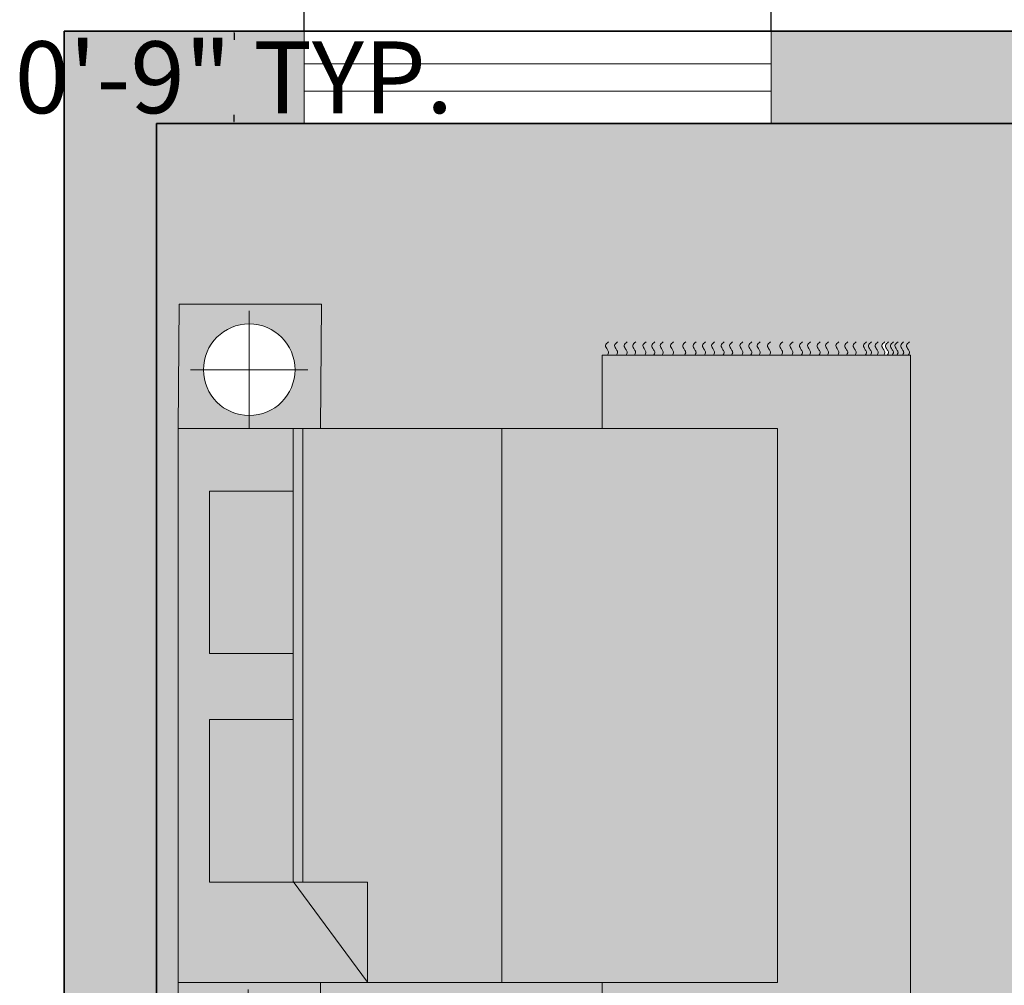
# Model space of a CAD drawing. Units: inches. Extents: x 1316 to 1777, y 813 to 1650.
# Tile 12 of 22: x 1373 to 1469, y 1482 to 1576. Entities that reach past the tile are written whole.
import ezdxf

# ---------------------------------------------------------------- set-up
doc = ezdxf.new("R2010")
doc.units = ezdxf.units.IN
doc.header["$MEASUREMENT"] = 0
for name, color, linetype, lineweight in [('A-ANNO-DIMS', 2, 'Continuous', 18), ('A-FURN-PATT', 23, 'Continuous', 13), ('A-WALL-PATT', 250, 'Continuous', 13), ('furniture', 23, 'Continuous', 18), ('walls', 250, 'Continuous', 35), ('windows', 141, 'Continuous', 18)]:
    doc.layers.add(name, color=color, linetype=linetype, lineweight=lineweight)
doc.layers.add('A-FLOR-PATT', color=254, linetype='Continuous', lineweight=13, true_color=0xfeeab9)
doc.styles.get("Standard").update_dxf_attribs({"font": 'arial.ttf'})
doc.dimstyles.get("Standard").update_dxf_attribs({"dimtxt": 7, "dimasz": 0.18, "dimexe": 0.18, "dimexo": 0.0625, "dimgap": 0.09, "dimtad": 0, "dimtih": 1, "dimtoh": 1, "dimzin": 0, "dimdsep": 46, "dimlunit": 3, "dimtxsty": 'Standard', "dimcen": 0.09, "dimadec": 0, "dimazin": 0, "dimtfac": 1, "dimtofl": 0, "dimtmove": 0, "dimatfit": 3, "dimfxl": 1, "dimtolj": 1, "dimtzin": 0, "dimarcsym": 0})

# ---------------------------------------------------------------- blocks, each defined once
blk = doc.blocks.new('CARPET')
at = {"layer": 'furniture'}
for p, q in [((-51.53, -98.11), (-51.53, -55.12)), ((-51.53, -55.12), (-41.27, -55.12)), ((36, -55.12), (51.55, -55.12)), ((51.55, -55.12), (51.55, -98.11)), ((51.55, -98.11), (-51.53, -98.11))]:
    blk.add_line(p, q, dxfattribs=at)
for points, knots in [([(-53.37, -55.99), (-53.22, -55.8), (-52.9, -55.41), (-52.34, -55.8), (-51.89, -56.08), (-51.65, -55.91), (-51.53, -55.83)], [0, 0, 0, 0, 0.653278, 1.290138, 1.740457, 2.114451, 2.114451, 2.114451, 2.114451]), ([(53.37, -55.99), (53.22, -55.8), (52.9, -55.41), (52.34, -55.8), (51.89, -56.08), (51.65, -55.91), (51.53, -55.83)], [0, 0, 0, 0, 0.653278, 1.290138, 1.740457, 2.114451, 2.114451, 2.114451, 2.114451]), ([(-53.37, -57.26), (-53.22, -57.07), (-52.9, -56.67), (-52.34, -57.07), (-51.89, -57.35), (-51.65, -57.17), (-51.53, -57.1)], [0, 0, 0, 0, 0.653278, 1.290138, 1.740457, 2.114451, 2.114451, 2.114451, 2.114451]), ([(53.37, -57.26), (53.22, -57.07), (52.9, -56.67), (52.34, -57.07), (51.89, -57.35), (51.65, -57.17), (51.53, -57.1)], [0, 0, 0, 0, 0.653278, 1.290138, 1.740457, 2.114451, 2.114451, 2.114451, 2.114451]), ([(-53.37, -58.59), (-53.22, -58.4), (-52.9, -58.01), (-52.34, -58.4), (-51.89, -58.68), (-51.65, -58.5), (-51.53, -58.43)], [0, 0, 0, 0, 0.653278, 1.290138, 1.740457, 2.114451, 2.114451, 2.114451, 2.114451]), ([(53.37, -58.59), (53.22, -58.4), (52.9, -58.01), (52.34, -58.4), (51.89, -58.68), (51.65, -58.5), (51.53, -58.43)], [0, 0, 0, 0, 0.653278, 1.290138, 1.740457, 2.114451, 2.114451, 2.114451, 2.114451]), ([(-53.37, -59.78), (-53.22, -59.58), (-52.9, -59.19), (-52.34, -59.58), (-51.89, -59.86), (-51.65, -59.69), (-51.53, -59.61)], [0, 0, 0, 0, 0.653278, 1.290138, 1.740457, 2.114451, 2.114451, 2.114451, 2.114451]), ([(53.37, -59.78), (53.22, -59.58), (52.9, -59.19), (52.34, -59.58), (51.89, -59.86), (51.65, -59.69), (51.53, -59.61)], [0, 0, 0, 0, 0.653278, 1.290138, 1.740457, 2.114451, 2.114451, 2.114451, 2.114451]), ([(-53.37, -61.22), (-53.22, -61.02), (-52.9, -60.63), (-52.34, -61.02), (-51.89, -61.3), (-51.65, -61.13), (-51.53, -61.05)], [0, 0, 0, 0, 0.653278, 1.290138, 1.740457, 2.114451, 2.114451, 2.114451, 2.114451]), ([(53.37, -61.22), (53.22, -61.02), (52.9, -60.63), (52.34, -61.02), (51.89, -61.3), (51.65, -61.13), (51.53, -61.05)], [0, 0, 0, 0, 0.653278, 1.290138, 1.740457, 2.114451, 2.114451, 2.114451, 2.114451]), ([(-53.37, -62.44), (-53.22, -62.25), (-52.9, -61.86), (-52.34, -62.25), (-51.89, -62.53), (-51.65, -62.36), (-51.53, -62.28)], [0, 0, 0, 0, 0.653278, 1.290138, 1.740457, 2.114451, 2.114451, 2.114451, 2.114451]), ([(-53.37, -63.63), (-53.22, -63.43), (-52.9, -63.04), (-52.34, -63.43), (-51.89, -63.72), (-51.65, -63.54), (-51.53, -63.46)], [0, 0, 0, 0, 0.653278, 1.290138, 1.740457, 2.114451, 2.114451, 2.114451, 2.114451]), ([(53.37, -62.44), (53.22, -62.25), (52.9, -61.86), (52.34, -62.25), (51.89, -62.53), (51.65, -62.36), (51.53, -62.28)], [0, 0, 0, 0, 0.653278, 1.290138, 1.740457, 2.114451, 2.114451, 2.114451, 2.114451]), ([(53.37, -63.63), (53.22, -63.43), (52.9, -63.04), (52.34, -63.43), (51.89, -63.72), (51.65, -63.54), (51.53, -63.46)], [0, 0, 0, 0, 0.653278, 1.290138, 1.740457, 2.114451, 2.114451, 2.114451, 2.114451]), ([(-53.37, -65.07), (-53.22, -64.87), (-52.9, -64.48), (-52.34, -64.87), (-51.89, -65.15), (-51.65, -64.98), (-51.53, -64.9)], [0, 0, 0, 0, 0.653278, 1.290138, 1.740457, 2.114451, 2.114451, 2.114451, 2.114451]), ([(53.37, -65.07), (53.22, -64.87), (52.9, -64.48), (52.34, -64.87), (51.89, -65.15), (51.65, -64.98), (51.53, -64.9)], [0, 0, 0, 0, 0.653278, 1.290138, 1.740457, 2.114451, 2.114451, 2.114451, 2.114451]), ([(-53.37, -66.76), (-53.22, -66.56), (-52.9, -66.17), (-52.34, -66.56), (-51.89, -66.84), (-51.65, -66.67), (-51.53, -66.59)], [0, 0, 0, 0, 0.653278, 1.290138, 1.740457, 2.114451, 2.114451, 2.114451, 2.114451]), ([(53.37, -66.76), (53.22, -66.56), (52.9, -66.17), (52.34, -66.56), (51.89, -66.84), (51.65, -66.67), (51.53, -66.59)], [0, 0, 0, 0, 0.653278, 1.290138, 1.740457, 2.114451, 2.114451, 2.114451, 2.114451]), ([(-53.37, -68.2), (-53.22, -68), (-52.9, -67.61), (-52.34, -68), (-51.89, -68.28), (-51.65, -68.11), (-51.53, -68.03)], [0, 0, 0, 0, 0.653278, 1.290138, 1.740457, 2.114451, 2.114451, 2.114451, 2.114451]), ([(53.37, -68.2), (53.22, -68), (52.9, -67.61), (52.34, -68), (51.89, -68.28), (51.65, -68.11), (51.53, -68.03)], [0, 0, 0, 0, 0.653278, 1.290138, 1.740457, 2.114451, 2.114451, 2.114451, 2.114451]), ([(-53.37, -69.53), (-53.22, -69.33), (-52.9, -68.94), (-52.34, -69.33), (-51.89, -69.61), (-51.65, -69.44), (-51.53, -69.36)], [0, 0, 0, 0, 0.653278, 1.290138, 1.740457, 2.114451, 2.114451, 2.114451, 2.114451]), ([(53.37, -69.53), (53.22, -69.33), (52.9, -68.94), (52.34, -69.33), (51.89, -69.61), (51.65, -69.44), (51.53, -69.36)], [0, 0, 0, 0, 0.653278, 1.290138, 1.740457, 2.114451, 2.114451, 2.114451, 2.114451]), ([(-53.37, -70.79), (-53.22, -70.6), (-52.9, -70.21), (-52.34, -70.6), (-51.89, -70.88), (-51.65, -70.7), (-51.53, -70.63)], [0, 0, 0, 0, 0.653278, 1.290138, 1.740457, 2.114451, 2.114451, 2.114451, 2.114451]), ([(53.37, -70.79), (53.22, -70.6), (52.9, -70.21), (52.34, -70.6), (51.89, -70.88), (51.65, -70.7), (51.53, -70.63)], [0, 0, 0, 0, 0.653278, 1.290138, 1.740457, 2.114451, 2.114451, 2.114451, 2.114451]), ([(-53.37, -72.12), (-53.22, -71.93), (-52.9, -71.54), (-52.34, -71.93), (-51.89, -72.21), (-51.65, -72.04), (-51.53, -71.96)], [0, 0, 0, 0, 0.653278, 1.290138, 1.740457, 2.114451, 2.114451, 2.114451, 2.114451]), ([(53.37, -72.12), (53.22, -71.93), (52.9, -71.54), (52.34, -71.93), (51.89, -72.21), (51.65, -72.04), (51.53, -71.96)], [0, 0, 0, 0, 0.653278, 1.290138, 1.740457, 2.114451, 2.114451, 2.114451, 2.114451]), ([(-53.37, -73.31), (-53.22, -73.11), (-52.9, -72.72), (-52.34, -73.11), (-51.89, -73.4), (-51.65, -73.22), (-51.53, -73.14)], [0, 0, 0, 0, 0.653278, 1.290138, 1.740457, 2.114451, 2.114451, 2.114451, 2.114451]), ([(53.37, -73.31), (53.22, -73.11), (52.9, -72.72), (52.34, -73.11), (51.89, -73.4), (51.65, -73.22), (51.53, -73.14)], [0, 0, 0, 0, 0.653278, 1.290138, 1.740457, 2.114451, 2.114451, 2.114451, 2.114451]), ([(-53.37, -74.75), (-53.22, -74.55), (-52.9, -74.16), (-52.34, -74.55), (-51.89, -74.83), (-51.65, -74.66), (-51.53, -74.58)], [0, 0, 0, 0, 0.653278, 1.290138, 1.740457, 2.114451, 2.114451, 2.114451, 2.114451]), ([(-53.37, -75.98), (-53.22, -75.78), (-52.9, -75.39), (-52.34, -75.78), (-51.89, -76.06), (-51.65, -75.89), (-51.53, -75.81)], [0, 0, 0, 0, 0.653278, 1.290138, 1.740457, 2.114451, 2.114451, 2.114451, 2.114451]), ([(53.37, -74.75), (53.22, -74.55), (52.9, -74.16), (52.34, -74.55), (51.89, -74.83), (51.65, -74.66), (51.53, -74.58)], [0, 0, 0, 0, 0.653278, 1.290138, 1.740457, 2.114451, 2.114451, 2.114451, 2.114451]), ([(53.37, -75.98), (53.22, -75.78), (52.9, -75.39), (52.34, -75.78), (51.89, -76.06), (51.65, -75.89), (51.53, -75.81)], [0, 0, 0, 0, 0.653278, 1.290138, 1.740457, 2.114451, 2.114451, 2.114451, 2.114451]), ([(-53.37, -77.16), (-53.22, -76.96), (-52.9, -76.57), (-52.34, -76.96), (-51.89, -77.25), (-51.65, -77.07), (-51.53, -76.99)], [0, 0, 0, 0, 0.653278, 1.290138, 1.740457, 2.114451, 2.114451, 2.114451, 2.114451]), ([(53.37, -77.16), (53.22, -76.96), (52.9, -76.57), (52.34, -76.96), (51.89, -77.25), (51.65, -77.07), (51.53, -76.99)], [0, 0, 0, 0, 0.653278, 1.290138, 1.740457, 2.114451, 2.114451, 2.114451, 2.114451]), ([(-53.37, -78.6), (-53.22, -78.4), (-52.9, -78.01), (-52.34, -78.4), (-51.89, -78.68), (-51.65, -78.51), (-51.53, -78.43)], [0, 0, 0, 0, 0.653278, 1.290138, 1.740457, 2.114451, 2.114451, 2.114451, 2.114451]), ([(53.37, -78.6), (53.22, -78.4), (52.9, -78.01), (52.34, -78.4), (51.89, -78.68), (51.65, -78.51), (51.53, -78.43)], [0, 0, 0, 0, 0.653278, 1.290138, 1.740457, 2.114451, 2.114451, 2.114451, 2.114451]), ([(-53.37, -80.29), (-53.22, -80.09), (-52.9, -79.7), (-52.34, -80.09), (-51.89, -80.37), (-51.65, -80.2), (-51.53, -80.12)], [0, 0, 0, 0, 0.653278, 1.290138, 1.740457, 2.114451, 2.114451, 2.114451, 2.114451]), ([(53.37, -80.29), (53.22, -80.09), (52.9, -79.7), (52.34, -80.09), (51.89, -80.37), (51.65, -80.2), (51.53, -80.12)], [0, 0, 0, 0, 0.653278, 1.290138, 1.740457, 2.114451, 2.114451, 2.114451, 2.114451]), ([(-53.37, -81.73), (-53.22, -81.53), (-52.9, -81.14), (-52.34, -81.53), (-51.89, -81.81), (-51.65, -81.64), (-51.53, -81.56)], [0, 0, 0, 0, 0.653278, 1.290138, 1.740457, 2.114451, 2.114451, 2.114451, 2.114451]), ([(53.37, -81.73), (53.22, -81.53), (52.9, -81.14), (52.34, -81.53), (51.89, -81.81), (51.65, -81.64), (51.53, -81.56)], [0, 0, 0, 0, 0.653278, 1.290138, 1.740457, 2.114451, 2.114451, 2.114451, 2.114451]), ([(-53.37, -83.06), (-53.22, -82.86), (-52.9, -82.47), (-52.34, -82.86), (-51.89, -83.14), (-51.65, -82.97), (-51.53, -82.89)], [0, 0, 0, 0, 0.653278, 1.290138, 1.740457, 2.114451, 2.114451, 2.114451, 2.114451]), ([(-53.37, -84.18), (-53.22, -83.99), (-52.9, -83.6), (-52.34, -83.99), (-51.89, -84.27), (-51.65, -84.09), (-51.53, -84.02)], [0, 0, 0, 0, 0.653278, 1.290138, 1.740457, 2.114451, 2.114451, 2.114451, 2.114451]), ([(53.37, -83.06), (53.22, -82.86), (52.9, -82.47), (52.34, -82.86), (51.89, -83.14), (51.65, -82.97), (51.53, -82.89)], [0, 0, 0, 0, 0.653278, 1.290138, 1.740457, 2.114451, 2.114451, 2.114451, 2.114451]), ([(53.37, -84.18), (53.22, -83.99), (52.9, -83.6), (52.34, -83.99), (51.89, -84.27), (51.65, -84.09), (51.53, -84.02)], [0, 0, 0, 0, 0.653278, 1.290138, 1.740457, 2.114451, 2.114451, 2.114451, 2.114451]), ([(-53.37, -85.51), (-53.22, -85.32), (-52.9, -84.93), (-52.34, -85.32), (-51.89, -85.6), (-51.65, -85.42), (-51.53, -85.35)], [0, 0, 0, 0, 0.653278, 1.290138, 1.740457, 2.114451, 2.114451, 2.114451, 2.114451]), ([(53.37, -85.51), (53.22, -85.32), (52.9, -84.93), (52.34, -85.32), (51.89, -85.6), (51.65, -85.42), (51.53, -85.35)], [0, 0, 0, 0, 0.653278, 1.290138, 1.740457, 2.114451, 2.114451, 2.114451, 2.114451]), ([(-53.37, -86.7), (-53.22, -86.5), (-52.9, -86.11), (-52.34, -86.5), (-51.89, -86.78), (-51.65, -86.61), (-51.53, -86.53)], [0, 0, 0, 0, 0.653278, 1.290138, 1.740457, 2.114451, 2.114451, 2.114451, 2.114451]), ([(53.37, -86.7), (53.22, -86.5), (52.9, -86.11), (52.34, -86.5), (51.89, -86.78), (51.65, -86.61), (51.53, -86.53)], [0, 0, 0, 0, 0.653278, 1.290138, 1.740457, 2.114451, 2.114451, 2.114451, 2.114451]), ([(-53.37, -88.14), (-53.22, -87.94), (-52.9, -87.55), (-52.34, -87.94), (-51.89, -88.22), (-51.65, -88.05), (-51.53, -87.97)], [0, 0, 0, 0, 0.653278, 1.290138, 1.740457, 2.114451, 2.114451, 2.114451, 2.114451]), ([(53.37, -88.14), (53.22, -87.94), (52.9, -87.55), (52.34, -87.94), (51.89, -88.22), (51.65, -88.05), (51.53, -87.97)], [0, 0, 0, 0, 0.653278, 1.290138, 1.740457, 2.114451, 2.114451, 2.114451, 2.114451]), ([(-53.37, -89.36), (-53.22, -89.17), (-52.9, -88.78), (-52.34, -89.17), (-51.89, -89.45), (-51.65, -89.28), (-51.53, -89.2)], [0, 0, 0, 0, 0.653278, 1.290138, 1.740457, 2.114451, 2.114451, 2.114451, 2.114451]), ([(53.37, -89.36), (53.22, -89.17), (52.9, -88.78), (52.34, -89.17), (51.89, -89.45), (51.65, -89.28), (51.53, -89.2)], [0, 0, 0, 0, 0.653278, 1.290138, 1.740457, 2.114451, 2.114451, 2.114451, 2.114451]), ([(-53.37, -90.55), (-53.22, -90.35), (-52.9, -89.96), (-52.34, -90.35), (-51.89, -90.64), (-51.65, -90.46), (-51.53, -90.38)], [0, 0, 0, 0, 0.653278, 1.290138, 1.740457, 2.114451, 2.114451, 2.114451, 2.114451]), ([(53.37, -90.55), (53.22, -90.35), (52.9, -89.96), (52.34, -90.35), (51.9, -90.63), (51.66, -90.47), (51.55, -90.4)], [0, 0, 0, 0, 0.653278, 1.290138, 1.740457, 2.0926, 2.0926, 2.0926, 2.0926]), ([(-53.37, -91.99), (-53.22, -91.79), (-52.9, -91.4), (-52.34, -91.79), (-51.89, -92.07), (-51.65, -91.9), (-51.53, -91.82)], [0, 0, 0, 0, 0.653278, 1.290138, 1.740457, 2.114451, 2.114451, 2.114451, 2.114451]), ([(53.37, -91.99), (53.22, -91.79), (52.9, -91.4), (52.34, -91.79), (51.9, -92.07), (51.66, -91.91), (51.55, -91.83)], [0, 0, 0, 0, 0.653278, 1.290138, 1.740457, 2.0926, 2.0926, 2.0926, 2.0926]), ([(-53.37, -92.69), (-53.22, -92.48), (-52.9, -92.08), (-52.35, -92.49), (-51.89, -92.77), (-51.65, -92.6), (-51.53, -92.52)], [0, 0, 0, 0, 0.663904, 1.307406, 1.757725, 2.131719, 2.131719, 2.131719, 2.131719]), ([(-53.37, -93.61), (-53.22, -93.42), (-52.9, -93.03), (-52.34, -93.42), (-51.89, -93.7), (-51.65, -93.52), (-51.53, -93.45)], [0, 0, 0, 0, 0.653278, 1.290138, 1.740457, 2.114451, 2.114451, 2.114451, 2.114451]), ([(53.37, -92.69), (53.22, -92.49), (52.9, -92.09), (52.34, -92.49), (51.9, -92.77), (51.66, -92.61), (51.55, -92.53)], [0, 0, 0, 0, 0.656792, 1.295826, 1.746145, 2.098292, 2.098292, 2.098292, 2.098292]), ([(53.37, -93.66), (53.22, -93.46), (52.9, -93.07), (52.34, -93.46), (51.9, -93.74), (51.66, -93.58), (51.55, -93.5)], [0, 0, 0, 0, 0.653278, 1.290138, 1.740457, 2.0926, 2.0926, 2.0926, 2.0926]), ([(-53.37, -94.55), (-53.22, -94.35), (-52.9, -93.96), (-52.34, -94.35), (-51.89, -94.63), (-51.65, -94.46), (-51.53, -94.38)], [0, 0, 0, 0, 0.653278, 1.290138, 1.740457, 2.114451, 2.114451, 2.114451, 2.114451]), ([(-53.37, -95.05), (-53.22, -94.85), (-52.9, -94.46), (-52.34, -94.85), (-51.89, -95.14), (-51.65, -94.96), (-51.53, -94.88)], [0, 0, 0, 0, 0.653278, 1.290138, 1.740457, 2.114451, 2.114451, 2.114451, 2.114451]), ([(53.37, -94.59), (53.22, -94.4), (52.9, -94.01), (52.34, -94.4), (51.9, -94.68), (51.66, -94.51), (51.55, -94.44)], [0, 0, 0, 0, 0.653278, 1.290138, 1.740457, 2.0926, 2.0926, 2.0926, 2.0926]), ([(53.37, -95.1), (53.22, -94.9), (52.9, -94.51), (52.34, -94.9), (51.9, -95.18), (51.66, -95.02), (51.55, -94.94)], [0, 0, 0, 0, 0.653278, 1.290138, 1.740457, 2.0926, 2.0926, 2.0926, 2.0926]), ([(-53.37, -95.73), (-53.22, -95.54), (-52.9, -95.15), (-52.34, -95.54), (-51.89, -95.82), (-51.65, -95.65), (-51.53, -95.57)], [0, 0, 0, 0, 0.653278, 1.290138, 1.740457, 2.114451, 2.114451, 2.114451, 2.114451]), ([(-53.37, -96.38), (-53.22, -96.18), (-52.9, -95.79), (-52.34, -96.18), (-51.89, -96.47), (-51.65, -96.29), (-51.53, -96.21)], [0, 0, 0, 0, 0.653278, 1.290138, 1.740457, 2.114451, 2.114451, 2.114451, 2.114451]), ([(53.37, -95.78), (53.22, -95.58), (52.9, -95.19), (52.34, -95.58), (51.89, -95.86), (51.65, -95.69), (51.53, -95.61)], [0, 0, 0, 0, 0.653278, 1.290138, 1.740457, 2.114451, 2.114451, 2.114451, 2.114451]), ([(53.37, -96.43), (53.22, -96.23), (52.9, -95.84), (52.34, -96.23), (51.89, -96.51), (51.65, -96.34), (51.53, -96.26)], [0, 0, 0, 0, 0.653278, 1.290138, 1.740457, 2.114451, 2.114451, 2.114451, 2.114451]), ([(-53.37, -97.17), (-53.22, -96.98), (-52.9, -96.59), (-52.34, -96.98), (-51.89, -97.26), (-51.65, -97.08), (-51.53, -97.01)], [0, 0, 0, 0, 0.653278, 1.290138, 1.740457, 2.114451, 2.114451, 2.114451, 2.114451]), ([(53.37, -97.22), (53.22, -97.02), (52.9, -96.63), (52.34, -97.02), (51.89, -97.3), (51.65, -97.13), (51.53, -97.05)], [0, 0, 0, 0, 0.653278, 1.290138, 1.740457, 2.114451, 2.114451, 2.114451, 2.114451]), ([(-53.37, -97.99), (-53.22, -97.79), (-52.9, -97.4), (-52.34, -97.79), (-51.89, -98.08), (-51.65, -97.9), (-51.53, -97.82)], [0, 0, 0, 0, 0.653278, 1.290138, 1.740457, 2.114451, 2.114451, 2.114451, 2.114451]), ([(53.37, -97.99), (53.22, -97.79), (52.9, -97.4), (52.34, -97.79), (51.89, -98.08), (51.65, -97.9), (51.53, -97.82)], [0, 0, 0, 0, 0.653278, 1.290138, 1.740457, 2.114451, 2.114451, 2.114451, 2.114451])]:
    blk.add_open_spline(points, degree=3, knots=knots, dxfattribs=at)
blk = doc.blocks.new('A$C58D270C6')
at = {"layer": 'furniture'}
for p, q in [((9.09, 124.13), (9.09, 108.87)), ((1.46, 116.5), (16.73, 116.5)), ((14.97, 94.84), (24.62, 107.92)), ((24.62, 94.93), (24.62, 107.92)), ((42.08, 108), (42.08, 36)), ((14.97, 94.93), (24.62, 94.93)), ((14.97, 94.84), (14.97, 36)), ((16.22, 94.93), (16.22, 36)), ((9.25, 36), (9.25, 20.74)), ((1.62, 28.37), (16.88, 28.37))]:
    blk.add_line(p, q, dxfattribs=at)
for points in [[(18.5, 108), (18.34, 124.13), (-0.16, 124.13), (0, 108)], [(0, 108), (77.91, 108), (77.91, 36), (0, 36)], [(4.09, 94.93), (14.97, 94.93), (14.97, 73.83), (4.09, 73.83)], [(4.09, 65.23), (14.97, 65.23), (14.97, 44.13), (4.09, 44.13)], [(18.65, 19.87), (18.5, 36), (0, 36), (0.16, 19.87)]]:
    blk.add_lwpolyline(points, close=True, dxfattribs=at)
for centre in [(9.09, 116.5), (9.25, 28.37)]:
    blk.add_circle(centre, 5.95, dxfattribs=at)
at = {"layer": 'furniture', "xscale": 0.9312884925094044, "yscale": 0.9312884925094044, "zscale": 0.9312884925094044, "rotation": 90}
blk.add_blockref('CARPET', (3.79, 74.47), dxfattribs=at)
blk = doc.blocks.new('WINDOW-45_5x9')
for p, q in [((0, 9), (0, 0)), ((45.51, 9), (0, 9)), ((45.51, 0), (45.51, 9)), ((0, 5.824), (45.51, 5.824)), ((45.51, 5.824), (45.51, 3.149)), ((45.51, 3.149), (0, 3.149)), ((0, 0), (45.51, 0))]:
    blk.add_line(p, q)
blk = doc.blocks.new('*D34')
at = {"layer": 'A-ANNO-DIMS', "color": 0, "lineweight": -2, "transparency": 16777216}
for p, q in [((1400.445, 1575.432), (1400.445, 1582.376)), ((1445.955, 1575.432), (1445.955, 1582.376)), ((1400.625, 1582.196), (1445.775, 1582.196)), ((1445.955, 1582.196), (1446.135, 1582.196))]:
    blk.add_line(p, q, dxfattribs=at)
at = {"layer": 'A-ANNO-DIMS', "color": 0, "transparency": 16777216}
for points in [[(1400.625, 1582.226), (1400.625, 1582.166), (1400.445, 1582.196)], [(1445.775, 1582.226), (1445.775, 1582.166), (1445.955, 1582.196)]]:
    blk.add_solid(points, dxfattribs=at)
at = {"layer": 'Defpoints', "color": 0, "transparency": 16777216}
for p in [(1445.955, 1582.196), (1400.445, 1575.369), (1445.955, 1575.369)]:
    blk.add_point(p, dxfattribs=at)
at = {"layer": 'A-ANNO-DIMS', "color": 0, "transparency": 16777216, "insert": (1498.67, 1582.196), "char_height": 7, "attachment_point": 5}
blk.add_mtext('\\A1;WINDOW 3\'-9 1/2" TYP.', dxfattribs=at)
blk = doc.blocks.new('*D35')
at = {"layer": 'A-ANNO-DIMS', "color": 0, "lineweight": -2, "transparency": 16777216}
for p, q in [((1400.382, 1575.369), (1393.438, 1575.369)), ((1393.618, 1575.189), (1393.618, 1574.533)), ((1393.618, 1566.549), (1393.618, 1567.205)), ((1400.382, 1566.369), (1393.438, 1566.369))]:
    blk.add_line(p, q, dxfattribs=at)
at = {"layer": 'A-ANNO-DIMS', "color": 0, "transparency": 16777216}
for points in [[(1393.588, 1575.189), (1393.648, 1575.189), (1393.618, 1575.369)], [(1393.588, 1566.549), (1393.648, 1566.549), (1393.618, 1566.369)]]:
    blk.add_solid(points, dxfattribs=at)
at = {"layer": 'Defpoints', "color": 0, "transparency": 16777216}
for p in [(1393.618, 1575.369), (1400.445, 1575.369), (1400.445, 1566.369)]:
    blk.add_point(p, dxfattribs=at)
at = {"layer": 'A-ANNO-DIMS', "color": 0, "transparency": 16777216, "insert": (1393.618, 1570.869), "char_height": 7, "attachment_point": 5}
blk.add_mtext('\\A1;0\'-9" TYP.', dxfattribs=at)

msp = doc.modelspace()

# ---------------------------------------------------------------- hatches: boundary and pattern name
at = {"layer": 'A-FLOR-PATT'}
h = msp.add_hatch(color=256, dxfattribs=at)
h.dxf.hatch_style = 1
h.paths.add_polyline_path([(1704.173, 1566.369), (1574.845, 1566.369), (1574.845, 1434.369), (1704.173, 1434.369)])
h.paths.add_polyline_path([(1630.932, 1542.856), (1660.956, 1542.856), (1660.956, 1535.716), (1688.427, 1535.716), (1688.322, 1546.604), (1686.085, 1547.859), (1686.091, 1547.88), (1685.166, 1550.963), (1681.619, 1555.397), (1678.246, 1552.474), (1678.253, 1552.433), (1678.187, 1552.423), (1681.619, 1555.397), (1683.601, 1556.058), (1683.639, 1556.172), (1683.764, 1556.112), (1686.94, 1557.171), (1688.039, 1558.585), (1688.034, 1558.699), (1688.108, 1558.672), (1686.969, 1557.208), (1686.965, 1557.18), (1681.619, 1555.397), (1682.039, 1554.872), (1682.12, 1554.846), (1682.107, 1554.788), (1685.145, 1550.989), (1685.188, 1550.977), (1685.173, 1550.941), (1685.764, 1548.971), (1688.364, 1547.814), (1702.185, 1547.814), (1702.301, 1535.716), (1702.301, 1481.716), (1702.418, 1469.617), (1688.544, 1469.617), (1688.427, 1481.716), (1660.956, 1481.716), (1660.956, 1470.853), (1630.932, 1470.853)], flags=16)
h.paths.add_polyline_path([(1624.931, 1450.279), (1703.919, 1450.279), (1703.919, 1436.32), (1703.919, 1435.026), (1624.931, 1435.026), (1624.931, 1435.469)], flags=16)
h.paths.add_polyline_path([(1624.931, 1443.714), (1625.995, 1443.714), (1625.995, 1449.229), (1626.752, 1449.229), (1626.752, 1443.714), (1628.114, 1443.714), (1628.114, 1449.229), (1628.871, 1449.229), (1628.871, 1443.714), (1630.502, 1443.714), (1630.502, 1449.229), (1631.259, 1449.229), (1631.259, 1443.714), (1632.968, 1443.714), (1632.968, 1449.229), (1633.724, 1449.229), (1633.724, 1443.714), (1638.318, 1443.714), (1641.013, 1449.6), (1641.689, 1449.29), (1639.136, 1443.714), (1640.128, 1443.714), (1642.823, 1449.6), (1643.499, 1449.29), (1640.945, 1443.714), (1642.323, 1443.714), (1645.018, 1449.6), (1645.694, 1449.29), (1643.141, 1443.714), (1647.035, 1443.714), (1647.035, 1449.229), (1647.792, 1449.229), (1647.792, 1443.714), (1649.606, 1443.714), (1649.606, 1449.229), (1650.363, 1449.229), (1650.363, 1443.714), (1652.865, 1443.714), (1652.865, 1449.229), (1653.621, 1449.229), (1653.621, 1443.714), (1657.035, 1443.714), (1657.035, 1449.229), (1657.792, 1449.229), (1657.792, 1443.714), (1660.083, 1443.714), (1660.083, 1449.229), (1660.839, 1449.229), (1660.839, 1443.714), (1662.605, 1443.714), (1662.605, 1449.229), (1663.362, 1449.229), (1663.362, 1443.714), (1667.702, 1443.714), (1667.702, 1449.229), (1668.459, 1449.229), (1668.459, 1443.714), (1671.655, 1443.714), (1670.316, 1449.229), (1671.051, 1449.407), (1672.434, 1443.714), (1679.696, 1443.714), (1680.179, 1449.244), (1680.933, 1449.178), (1680.455, 1443.714), (1683.5, 1443.714), (1682.225, 1448.723), (1682.959, 1448.91), (1684.281, 1443.714), (1688.219, 1443.714), (1688.219, 1449.229), (1688.976, 1449.229), (1688.976, 1443.714), (1690.482, 1443.714), (1690.482, 1449.229), (1691.239, 1449.229), (1691.239, 1443.714), (1692.488, 1443.714), (1692.488, 1449.229), (1693.245, 1449.229), (1693.245, 1443.714), (1695.009, 1443.714), (1695.009, 1449.229), (1695.766, 1449.229), (1695.766, 1443.714), (1701.029, 1443.714), (1700.875, 1443.379), (1695.766, 1443.379), (1695.766, 1435.872), (1695.009, 1435.872), (1695.009, 1443.379), (1693.245, 1443.379), (1693.245, 1435.872), (1692.488, 1435.872), (1692.488, 1443.379), (1691.239, 1443.379), (1691.239, 1435.872), (1690.482, 1435.872), (1690.482, 1443.379), (1688.976, 1443.379), (1688.976, 1435.872), (1688.219, 1435.872), (1688.219, 1443.379), (1684.366, 1443.379), (1686.252, 1435.965), (1685.518, 1435.779), (1683.585, 1443.379), (1680.426, 1443.379), (1679.77, 1435.872), (1679.016, 1435.938), (1679.666, 1443.379), (1677.602, 1443.379), (1677.602, 1435.46), (1676.845, 1435.46), (1676.845, 1443.379), (1672.515, 1443.379), (1674.202, 1436.427), (1673.467, 1436.249), (1671.736, 1443.379), (1668.459, 1443.379), (1668.459, 1435.872), (1667.702, 1435.872), (1667.702, 1443.379), (1663.362, 1443.379), (1663.362, 1435.872), (1662.605, 1435.872), (1662.605, 1443.379), (1660.839, 1443.379), (1660.839, 1435.872), (1660.083, 1435.872), (1660.083, 1443.379), (1657.792, 1443.379), (1657.792, 1435.872), (1657.035, 1435.872), (1657.035, 1443.379), (1653.621, 1443.379), (1653.621, 1435.872), (1652.865, 1435.872), (1652.865, 1443.379), (1650.363, 1443.379), (1650.363, 1435.872), (1649.606, 1435.872), (1649.606, 1443.379), (1647.792, 1443.379), (1647.792, 1435.872), (1647.035, 1435.872), (1647.035, 1443.379), (1642.988, 1443.379), (1639.39, 1435.522), (1638.715, 1435.832), (1642.17, 1443.379), (1640.792, 1443.379), (1637.195, 1435.522), (1636.519, 1435.832), (1639.974, 1443.379), (1638.983, 1443.379), (1635.385, 1435.522), (1634.709, 1435.832), (1638.165, 1443.379), (1633.724, 1443.379), (1633.724, 1435.872), (1632.968, 1435.872), (1632.968, 1443.379), (1631.259, 1443.379), (1631.259, 1435.872), (1630.502, 1435.872), (1630.502, 1443.379), (1628.871, 1443.379), (1628.871, 1435.872), (1628.114, 1435.872), (1628.114, 1443.379), (1626.752, 1443.379), (1626.752, 1435.872), (1625.995, 1435.872), (1625.995, 1443.379), (1624.931, 1443.379)], flags=0)
h.paths.add_polyline_path([(1683.839, 1491.517), (1691.022, 1491.517), (1691.071, 1491.582), (1691.071, 1529.618), (1699.231, 1529.618), (1699.231, 1513.795), (1691.071, 1513.795), (1691.071, 1507.34), (1699.231, 1507.34), (1699.231, 1491.517), (1691.022, 1491.517), (1683.839, 1481.774)], flags=0)
h.paths.add_polyline_path([(1691.015, 1475.341, -1), (1699.947, 1475.341, -1)], flags=0)
h.paths.add_polyline_path([(1690.898, 1541.439, -1), (1699.83, 1541.439, -1)], flags=0)
h.paths.add_polyline_path([(1505.845, 1469.591), (1505.845, 1566.369), (1386.064, 1566.369), (1386.064, 1450.329), (1465.697, 1450.329), (1465.697, 1449.245), (1466.177, 1449.025), (1465.697, 1447.977), (1465.697, 1436.055), (1465.697, 1434.369), (1505.845, 1434.369), (1505.845, 1440.551), (1476.949, 1440.551), (1476.949, 1441.822), (1476.977, 1441.822, -0.400014)])
edge = h.paths.add_edge_path(flags=16)
edge.add_spline(control_points=[(1456.973, 1471.794), (1457.023, 1471.721), (1457.138, 1471.554), (1456.942, 1471.242), (1456.67, 1470.851), (1456.943, 1470.632), (1457.081, 1470.522)], knot_values=[0, 0, 0, 0, 0.352144, 0.802463, 1.439322, 2.0926, 2.0926, 2.0926, 2.0926], degree=3, periodic=0)
edge.add_spline(control_points=[(1457.325, 1471.794), (1457.375, 1471.721), (1457.49, 1471.554), (1457.294, 1471.242), (1457.022, 1470.851), (1457.295, 1470.632), (1457.433, 1470.522)], knot_values=[0, 0, 0, 0, 0.352144, 0.802463, 1.439322, 2.0926, 2.0926, 2.0926, 2.0926], degree=3, periodic=0)
edge = h.paths.add_edge_path(flags=16)
edge.add_line((1429.513, 1471.794), (1429.513, 1482.657))
edge.add_line((1429.513, 1482.657), (1402.042, 1482.657))
edge.add_line((1402.042, 1482.657), (1401.925, 1470.559))
edge.add_line((1401.925, 1470.559), (1388.051, 1470.559))
edge.add_line((1388.051, 1470.559), (1388.167, 1482.657))
edge.add_line((1388.167, 1482.657), (1388.167, 1536.657))
edge.add_line((1388.167, 1536.657), (1388.284, 1548.755))
edge.add_line((1388.284, 1548.755), (1402.158, 1548.755))
edge.add_line((1402.158, 1548.755), (1402.042, 1536.657))
edge.add_line((1402.042, 1536.657), (1429.513, 1536.657))
edge.add_line((1429.513, 1536.657), (1429.513, 1543.797))
edge.add_line((1429.513, 1543.797), (1456.932, 1543.797))
edge.add_spline(control_points=[(1456.932, 1543.797), (1456.987, 1543.874), (1457.108, 1544.044), (1456.911, 1544.361), (1456.638, 1544.752), (1456.911, 1544.971), (1457.049, 1545.082)], knot_values=[0, 0, 0, 0, 0.373994, 0.824314, 1.461173, 2.114451, 2.114451, 2.114451, 2.114451], degree=3, periodic=0)
edge.add_spline(control_points=[(1457.401, 1545.082), (1457.263, 1544.971), (1456.99, 1544.752), (1457.263, 1544.361), (1457.46, 1544.044), (1457.339, 1543.874), (1457.284, 1543.797)], knot_values=[0, 0, 0, 0, 0.653278, 1.290138, 1.740457, 2.114451, 2.114451, 2.114451, 2.114451], degree=3, periodic=0)
edge.add_line((1457.284, 1543.797), (1459.536, 1543.797))
edge.add_line((1459.536, 1543.797), (1459.536, 1471.794))
edge.add_line((1459.536, 1471.794), (1429.513, 1471.794))
h.paths.add_polyline_path([(1406.63, 1482.715), (1399.446, 1492.458), (1399.398, 1492.458), (1391.238, 1492.458), (1391.238, 1508.281), (1399.398, 1508.281), (1399.398, 1514.736), (1391.238, 1514.736), (1391.238, 1530.559), (1399.398, 1530.559), (1399.398, 1492.524), (1399.446, 1492.458), (1406.63, 1492.458)], flags=0)
h.paths.add_polyline_path([(1399.454, 1476.282, -1), (1390.522, 1476.282, -1)], flags=0)
h.paths.add_polyline_path([(1390.638, 1542.38, -1), (1399.571, 1542.38, -1)], flags=0)
h.paths.add_polyline_path([(1487.293, 1548.286), (1487.08, 1548.252), (1487.104, 1547.964)], flags=16)
h.paths.add_polyline_path([(1491.493, 1552.843), (1490.887, 1552.654), (1490.949, 1552.372)], flags=16)
h.paths.add_polyline_path([(1489.966, 1554.409), (1489.859, 1554.561), (1489.718, 1554.445)], flags=16)
h.paths.add_polyline_path([(1497.301, 1546.483), (1497.294, 1546.462), (1497.309, 1546.453)], flags=16)
h.paths.add_polyline_path([(1496.386, 1549.553), (1492.828, 1554), (1492.655, 1554.939), (1492.454, 1555.029), (1492.589, 1555.296), (1491.806, 1559.547), (1491.869, 1559.506), (1491.824, 1559.451), (1492.828, 1554), (1494.81, 1554.661), (1494.848, 1554.774), (1494.973, 1554.715), (1496.01, 1555.061), (1496.078, 1555.314), (1496.341, 1555.171), (1498.15, 1555.774), (1499.249, 1557.187), (1499.243, 1557.301), (1499.317, 1557.275), (1498.179, 1555.811), (1498.174, 1555.782), (1492.828, 1554), (1493.249, 1553.474), (1493.33, 1553.449), (1493.316, 1553.39), (1495.203, 1551.032), (1495.702, 1550.957), (1495.574, 1550.568), (1496.354, 1549.592), (1496.397, 1549.58)], flags=16)
h.paths.add_polyline_path([(1486.021, 1555.224), (1485.958, 1555.549), (1483.595, 1557.912), (1483.28, 1557.859), (1483.243, 1558.264), (1486.27, 1555.237)], flags=16)
h.paths.add_polyline_path([(1505.845, 1469.591, 0.400014), (1476.977, 1441.822), (1505.845, 1441.822)], flags=17)
at = {"layer": 'A-FURN-PATT'}
h = msp.add_hatch(color=256, dxfattribs=at)
h.dxf.hatch_style = 1
h.paths.add_polyline_path([(1429.479, 1448.964), (1430.236, 1448.964), (1430.236, 1443.449), (1433.432, 1443.449), (1432.094, 1448.964), (1432.829, 1449.142), (1434.211, 1443.449), (1441.473, 1443.449), (1441.957, 1448.979), (1442.711, 1448.913), (1442.233, 1443.449), (1445.277, 1443.449), (1444.003, 1448.458), (1444.736, 1448.645), (1446.058, 1443.449), (1449.997, 1443.449), (1449.997, 1448.964), (1450.753, 1448.964), (1450.753, 1443.449), (1452.259, 1443.449), (1452.259, 1448.964), (1453.016, 1448.964), (1453.016, 1443.449), (1454.266, 1443.449), (1454.266, 1448.964), (1455.022, 1448.964), (1455.022, 1443.449), (1456.787, 1443.449), (1456.787, 1448.964), (1457.544, 1448.964), (1457.544, 1443.449), (1462.806, 1443.449), (1465.501, 1449.335), (1465.697, 1449.245), (1465.697, 1450.014), (1386.708, 1450.014), (1386.708, 1443.449), (1387.773, 1443.449), (1387.773, 1448.964), (1388.529, 1448.964), (1388.529, 1443.449), (1389.891, 1443.449), (1389.891, 1448.964), (1390.648, 1448.964), (1390.648, 1443.449), (1392.28, 1443.449), (1392.28, 1448.964), (1393.037, 1448.964), (1393.037, 1443.449), (1394.745, 1443.449), (1394.745, 1448.964), (1395.502, 1448.964), (1395.502, 1443.449), (1400.096, 1443.449), (1402.791, 1449.335), (1403.467, 1449.025), (1400.913, 1443.449), (1401.905, 1443.449), (1404.6, 1449.335), (1405.276, 1449.025), (1402.723, 1443.449), (1404.101, 1443.449), (1406.796, 1449.335), (1407.472, 1449.025), (1404.918, 1443.449), (1408.812, 1443.449), (1408.812, 1448.964), (1409.569, 1448.964), (1409.569, 1443.449), (1411.384, 1443.449), (1411.384, 1448.964), (1412.141, 1448.964), (1412.141, 1443.449), (1414.642, 1443.449), (1414.642, 1448.964), (1415.399, 1448.964), (1415.399, 1443.449), (1418.813, 1443.449), (1418.813, 1448.964), (1419.569, 1448.964), (1419.569, 1443.449), (1421.86, 1443.449), (1421.86, 1448.964), (1422.617, 1448.964), (1422.617, 1443.449), (1424.382, 1443.449), (1424.382, 1448.964), (1425.139, 1448.964), (1425.139, 1443.449), (1429.479, 1443.449)])
h.paths.add_polyline_path([(1429.479, 1443.114), (1425.139, 1443.114), (1425.139, 1435.607), (1424.382, 1435.607), (1424.382, 1443.114), (1422.617, 1443.114), (1422.617, 1435.607), (1421.86, 1435.607), (1421.86, 1443.114), (1419.569, 1443.114), (1419.569, 1435.607), (1418.813, 1435.607), (1418.813, 1443.114), (1415.399, 1443.114), (1415.399, 1435.607), (1414.642, 1435.607), (1414.642, 1443.114), (1412.141, 1443.114), (1412.141, 1435.607), (1411.384, 1435.607), (1411.384, 1443.114), (1409.569, 1443.114), (1409.569, 1435.607), (1408.812, 1435.607), (1408.812, 1443.114), (1404.765, 1443.114), (1401.168, 1435.258), (1400.492, 1435.567), (1403.948, 1443.114), (1402.57, 1443.114), (1398.972, 1435.258), (1398.296, 1435.567), (1401.752, 1443.114), (1400.76, 1443.114), (1397.163, 1435.258), (1396.487, 1435.567), (1399.943, 1443.114), (1395.502, 1443.114), (1395.502, 1435.607), (1394.745, 1435.607), (1394.745, 1443.114), (1393.037, 1443.114), (1393.037, 1435.607), (1392.28, 1435.607), (1392.28, 1443.114), (1390.648, 1443.114), (1390.648, 1435.607), (1389.891, 1435.607), (1389.891, 1443.114), (1388.529, 1443.114), (1388.529, 1435.607), (1387.773, 1435.607), (1387.773, 1443.114), (1386.708, 1443.114), (1386.708, 1436.055), (1386.708, 1435.204), (1386.708, 1434.762), (1465.697, 1434.762), (1465.697, 1447.977), (1459.873, 1435.258), (1459.197, 1435.567), (1462.653, 1443.114), (1457.544, 1443.114), (1457.544, 1435.607), (1456.787, 1435.607), (1456.787, 1443.114), (1455.022, 1443.114), (1455.022, 1435.607), (1454.266, 1435.607), (1454.266, 1443.114), (1453.016, 1443.114), (1453.016, 1435.607), (1452.259, 1435.607), (1452.259, 1443.114), (1450.753, 1443.114), (1450.753, 1435.607), (1449.997, 1435.607), (1449.997, 1443.114), (1446.143, 1443.114), (1448.029, 1435.7), (1447.296, 1435.514), (1445.362, 1443.114), (1442.204, 1443.114), (1441.547, 1435.607), (1440.793, 1435.673), (1441.444, 1443.114), (1439.379, 1443.114), (1439.379, 1435.195), (1438.623, 1435.195), (1438.623, 1443.114), (1434.292, 1443.114), (1435.98, 1436.163), (1435.245, 1435.984), (1433.514, 1443.114), (1430.236, 1443.114), (1430.236, 1435.607), (1429.479, 1435.607)])
h.paths.add_polyline_path([(1402.042, 1482.657), (1388.167, 1482.657), (1388.051, 1470.559), (1394.988, 1470.559), (1394.988, 1471.816, -0.414214), (1390.522, 1476.282, -1), (1399.454, 1476.282, -0.414214), (1394.988, 1471.816), (1394.988, 1470.559), (1401.925, 1470.559)])
h.paths.add_polyline_path([(1399.398, 1514.736), (1391.238, 1514.736), (1391.238, 1530.559), (1399.398, 1530.559), (1399.398, 1536.657), (1388.167, 1536.657), (1388.167, 1482.657), (1406.63, 1482.657), (1406.63, 1482.715), (1399.446, 1492.458), (1391.238, 1492.458), (1391.238, 1508.281), (1399.398, 1508.281)])
h.paths.add_polyline_path([(1399.571, 1542.38, -0.414214), (1395.105, 1537.914), (1395.105, 1536.657), (1402.042, 1536.657), (1402.158, 1548.755), (1388.284, 1548.755), (1388.167, 1536.657), (1395.105, 1536.657), (1395.105, 1537.914, -0.414214), (1390.638, 1542.38, -1)])
h = msp.add_hatch(color=256, dxfattribs=at)
h.dxf.hatch_style = 1
h.paths.add_polyline_path([(1399.398, 1508.281), (1391.238, 1508.281), (1391.238, 1492.458), (1399.398, 1492.458)])
h.paths.add_polyline_path([(1399.398, 1530.559), (1391.238, 1530.559), (1391.238, 1514.736), (1399.398, 1514.736)])
h.paths.add_polyline_path([(1459.536, 1543.797), (1429.513, 1543.797), (1429.513, 1536.657), (1446.596, 1536.657), (1446.596, 1482.657), (1429.513, 1482.657), (1429.513, 1471.794), (1459.536, 1471.794)])
h = msp.add_hatch(color=256, dxfattribs=at)
h.dxf.hatch_style = 1
h.paths.add_polyline_path([(1406.63, 1492.458), (1399.446, 1492.458), (1406.63, 1482.715)])
h.paths.add_polyline_path([(1400.33, 1536.657), (1399.398, 1536.657), (1399.398, 1492.524), (1399.446, 1492.458), (1400.33, 1492.458)])
h = msp.add_hatch(color=256, dxfattribs=at)
h.dxf.hatch_style = 1
h.paths.add_polyline_path([(1446.596, 1536.657), (1419.726, 1536.657), (1419.726, 1482.657), (1446.596, 1482.657)])
h.paths.add_polyline_path([(1419.726, 1536.657), (1400.33, 1536.657), (1400.33, 1492.458), (1406.63, 1492.458), (1406.63, 1482.657), (1419.726, 1482.657)])
at = {"layer": 'A-WALL-PATT'}
h = msp.add_hatch(color=256, dxfattribs=at)
h.dxf.hatch_style = 1
h.paths.add_polyline_path([(1713.173, 1281.369), (1656.173, 1281.369), (1656.173, 1298.258), (1651.673, 1298.258), (1651.673, 1281.369), (1567.673, 1281.369), (1567.673, 1266.995), (1572.173, 1266.995), (1572.173, 1276.869), (1704.173, 1276.869), (1704.173, 1132.869), (1608.64, 1132.869), (1608.64, 1123.869), (1704.173, 1123.869), (1704.173, 1040.173), (1652.869, 1040.173), (1652.869, 1031.173), (1713.173, 1031.173), (1713.173, 1040.173)])
h.paths.add_polyline_path([(1572.173, 1237.955), (1567.673, 1237.955), (1567.673, 1123.869), (1583.146, 1123.869), (1583.146, 1132.869), (1572.173, 1132.869)], flags=17)
h.paths.add_polyline_path([(1510.345, 1566.369), (1524.171, 1566.369), (1524.171, 1571.985), (1524.171, 1575.369), (1445.955, 1575.369), (1445.955, 1566.369), (1505.845, 1566.369), (1505.845, 1469.591), (1510.345, 1469.591), (1510.345, 1471.869), (1529.081, 1471.869), (1529.081, 1476.369), (1510.345, 1476.369)])
h.paths.add_polyline_path([(1609.722, 1575.369), (1545.119, 1575.369), (1545.119, 1566.369), (1570.345, 1566.369), (1570.345, 1476.369), (1562.477, 1476.369), (1562.477, 1471.869), (1570.345, 1471.869), (1570.345, 1469.591), (1574.845, 1469.591), (1574.845, 1566.369), (1609.722, 1566.369)])
h.paths.add_polyline_path([(1713.173, 1575.369), (1655.233, 1575.369), (1655.233, 1566.369), (1704.173, 1566.369), (1704.173, 1434.369), (1574.845, 1434.369), (1574.845, 1440.551), (1574.701, 1440.551), (1570.345, 1440.551), (1570.345, 1429.869), (1597.673, 1429.869), (1597.673, 1408.281), (1602.173, 1408.281), (1602.173, 1429.869), (1704.173, 1429.869), (1704.173, 1410.704), (1707.375, 1410.704), (1713.173, 1410.704)])
h.paths.add_polyline_path([(1713.173, 1383.676), (1704.173, 1383.676), (1704.173, 1369.869), (1602.173, 1369.869), (1602.173, 1379.241), (1597.673, 1379.241), (1597.673, 1365.369), (1713.173, 1365.369)])
h.paths.add_polyline_path([(1444.564, 1429.869), (1510.345, 1429.869), (1510.345, 1440.551), (1505.845, 1440.551), (1505.845, 1434.369), (1386.064, 1434.369), (1386.064, 1566.369), (1400.445, 1566.369), (1400.445, 1575.369), (1377.064, 1575.369), (1377.064, 1412.813), (1380.509, 1412.813), (1386.064, 1412.813), (1386.064, 1429.869), (1440.064, 1429.869), (1440.064, 1401.229), (1444.564, 1401.229)])
h.paths.add_polyline_path([(1444.564, 1372.189), (1440.064, 1372.189), (1440.064, 1369.869), (1386.064, 1369.869), (1386.064, 1378.758), (1377.064, 1378.758), (1377.064, 1349.201), (1381.118, 1349.201), (1386.064, 1349.201), (1386.064, 1365.369), (1440.064, 1365.369), (1440.064, 1322.882), (1444.564, 1322.882)])
h.paths.add_polyline_path([(1510.564, 1295.094), (1506.064, 1295.094), (1506.064, 1245.369), (1386.064, 1245.369), (1386.064, 1272.582), (1377.064, 1272.582), (1377.064, 1212.905), (1380.1, 1212.905), (1386.064, 1212.905), (1386.064, 1240.869), (1510.564, 1240.869)])
h.paths.add_polyline_path([(1386.064, 1163.761), (1377.064, 1163.761), (1377.064, 1063.869), (1419.363, 1063.869), (1419.363, 1072.869), (1386.064, 1072.869)])
h.paths.add_polyline_path([(1510.564, 1072.869), (1469.381, 1072.869), (1469.381, 1063.869), (1501.564, 1063.869), (1501.564, 1033.023), (1501.564, 1031.173), (1540.829, 1031.173), (1540.829, 1036.182, -0.029954), (1541.068, 1040.173), (1510.564, 1040.173)])
h.paths.add_polyline_path([(1607.369, 1040.173), (1574.225, 1040.173), (1574.225, 1036.182), (1574.225, 1031.173), (1607.369, 1031.173)], flags=17)
h.paths.add_polyline_path([(1637.054, 1040.173), (1624.706, 1040.173), (1624.706, 1031.173), (1637.054, 1031.173)], flags=17)

# ---------------------------------------------------------------- linework, layer by layer
at = {"layer": 'walls'}
for p, q in [((1377.064, 1575.369), (1713.173, 1575.369)), ((1377.064, 1575.369), (1377.064, 953.689)), ((1386.064, 1566.369), (1505.845, 1566.369)), ((1386.064, 1566.369), (1386.064, 1434.369))]:
    msp.add_line(p, q, dxfattribs=at)

# ---------------------------------------------------------------- block references
at = {"layer": 'furniture', "xscale": -0.7500000390647866, "yscale": 0.7500000390647866, "zscale": 0.7500000390647866, "rotation": 180}
msp.add_blockref('A$C58D270C6', (1388.167, 1563.657), dxfattribs=at)
at = {"layer": 'windows'}
msp.add_blockref('WINDOW-45_5x9', (1400.445, 1566.369), dxfattribs=at)

# ---------------------------------------------------------------- dimensions: what is measured, and where the dimension line sits
at = {"layer": 'A-ANNO-DIMS'}
dim = msp.add_linear_dim(base=(1445.955, 1582.196), p1=(1400.445, 1575.369), p2=(1445.955, 1575.369), text='WINDOW <> TYP.', dimstyle='Standard', override={"dimdec": 1, "dimlfac": 1, "dimrnd": 0, "dimzin": 1, "dimdsep": 46, "dimlunit": 4, "dimfrac": 2}, dxfattribs=at)
dim.commit()
dim.dimension.update_dxf_attribs({"geometry": '*D34', "text_midpoint": (1498.67, 1582.196)})
dim = msp.add_linear_dim(base=(1393.618, 1575.369), p1=(1400.445, 1566.369), p2=(1400.445, 1575.369), angle=90, text='<> TYP.', dimstyle='Standard', override={"dimdec": 1, "dimlfac": 1, "dimrnd": 0, "dimzin": 1, "dimdsep": 46, "dimlunit": 4, "dimfrac": 2}, dxfattribs=at)
dim.commit()
dim.dimension.update_dxf_attribs({"geometry": '*D35', "text_midpoint": (1393.618, 1570.869)})

doc.saveas('drawing.dxf')
